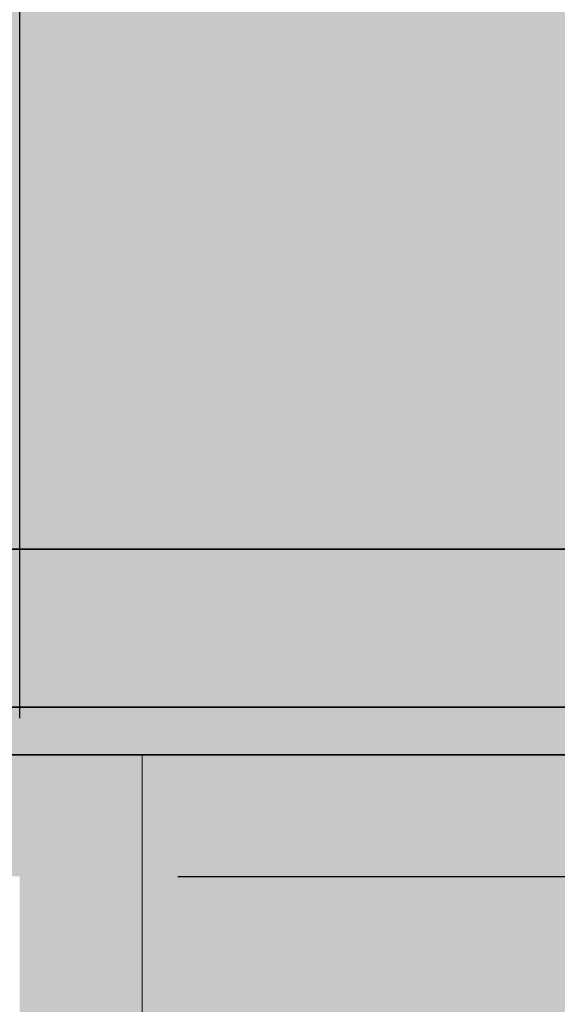
# Model space of a CAD drawing. Units: millimetres. Extents: x 130 to 1021, y 147 to 699.
# Tile 13 of 40: x 545 to 579, y 378 to 440. Entities that reach past the tile are written whole.
import ezdxf

# ---------------------------------------------------------------- set-up
doc = ezdxf.new("R2010")
doc.units = ezdxf.units.MM
doc.header["$MEASUREMENT"] = 0
for name, color, linetype, lineweight in [('A-ANNO-DIMS', 2, 'Continuous', 18), ('A-ELEV', 7, 'Continuous', 35), ('A-ELEV-PATT', 9, 'Continuous', 13), ('A-GLAZ', 4, 'Continuous', 18)]:
    doc.layers.add(name, color=color, linetype=linetype, lineweight=lineweight)
doc.styles.get("Standard").update_dxf_attribs({"font": 'arial.ttf'})
doc.dimstyles.get("Standard").update_dxf_attribs({"dimtxt": 20, "dimasz": 10, "dimexe": 10, "dimexo": 10, "dimgap": 5, "dimtad": 0, "dimtih": 1, "dimtoh": 1, "dimdec": 0, "dimzin": 0, "dimdsep": 46, "dimtxsty": 'Standard', "dimcen": 5, "dimadec": 0, "dimazin": 0, "dimtfac": 1, "dimtdec": 0, "dimtofl": 0, "dimtmove": 0, "dimatfit": 3, "dimfxl": 1, "dimtolj": 1, "dimtzin": 0, "dimarcsym": 0})

# ---------------------------------------------------------------- blocks, each defined once
blk = doc.blocks.new('*D7')
at = {"layer": 'A-ANNO-DIMS', "color": 0, "lineweight": -2, "transparency": 16777216}
for p, q in [((399.374, 349.447), (413.374, 349.447)), ((423.374, 349.447), (433.374, 349.447)), ((389.374, 344.547), (389.374, 339.447)), ((423.374, 344.547), (423.374, 339.447))]:
    blk.add_line(p, q, dxfattribs=at)
at = {"layer": 'A-ANNO-DIMS', "color": 0, "transparency": 16777216}
for points in [[(399.374, 351.114), (399.374, 347.781), (389.374, 349.447)], [(413.374, 351.114), (413.374, 347.781), (423.374, 349.447)]]:
    blk.add_solid(points, dxfattribs=at)
at = {"layer": 'Defpoints', "color": 0, "transparency": 16777216}
for p in [(389.374, 354.547), (423.374, 354.547), (423.374, 349.447)]:
    blk.add_point(p, dxfattribs=at)
at = {"layer": 'A-ANNO-DIMS', "color": 0, "transparency": 16777216, "insert": (582.037, 349.447), "char_height": 20, "attachment_point": 5}
blk.add_mtext('\\A1;DOOR PANEL 34 TYP.', dxfattribs=at)
blk = doc.blocks.new('*D11')
at = {"layer": 'A-ANNO-DIMS', "color": 0, "lineweight": -2, "transparency": 16777216}
for p, q in [((737.374, 648.699), (737.374, 149.739)), ((299.374, 566.947), (299.374, 149.739)), ((309.374, 159.739), (490.857, 159.739)), ((727.374, 159.739), (545.891, 159.739))]:
    blk.add_line(p, q, dxfattribs=at)
at = {"layer": 'A-ANNO-DIMS', "color": 0, "transparency": 16777216}
for points in [[(309.374, 161.406), (309.374, 158.073), (299.374, 159.739)], [(727.374, 161.406), (727.374, 158.073), (737.374, 159.739)]]:
    blk.add_solid(points, dxfattribs=at)
at = {"layer": 'Defpoints', "color": 0, "transparency": 16777216}
for p in [(737.374, 658.699), (299.374, 576.947), (737.374, 159.739)]:
    blk.add_point(p, dxfattribs=at)
at = {"layer": 'A-ANNO-DIMS', "color": 0, "transparency": 16777216, "insert": (518.374, 159.739), "char_height": 20, "attachment_point": 5}
blk.add_mtext('\\A1;438', dxfattribs=at)
blk = doc.blocks.new('*D22')
at = {"layer": 'A-ANNO-DIMS', "color": 0, "lineweight": -2, "transparency": 16777216}
for p, q in [((447.374, 656.947), (447.374, 696.247)), ((466.767, 403.947), (466.767, 696.247)), ((437.374, 686.247), (427.374, 686.247)), ((476.767, 686.247), (486.767, 686.247))]:
    blk.add_line(p, q, dxfattribs=at)
at = {"layer": 'A-ANNO-DIMS', "color": 0, "transparency": 16777216}
for points in [[(437.374, 687.914), (437.374, 684.581), (447.374, 686.247)], [(476.767, 687.914), (476.767, 684.581), (466.767, 686.247)]]:
    blk.add_solid(points, dxfattribs=at)
at = {"layer": 'Defpoints', "color": 0, "transparency": 16777216}
for p in [(466.767, 686.247), (447.374, 646.947), (466.767, 393.947)]:
    blk.add_point(p, dxfattribs=at)
at = {"layer": 'A-ANNO-DIMS', "color": 0, "transparency": 16777216, "insert": (532.34, 686.247), "char_height": 20, "attachment_point": 5}
blk.add_mtext('\\A1;19.393', dxfattribs=at)
blk = doc.blocks.new('*D23')
at = {"layer": 'A-ANNO-DIMS', "color": 0, "lineweight": -2, "transparency": 16777216}
for p, q in [((466.767, 403.947), (466.767, 696.247)), ((475.988, 209.039), (475.988, 696.247)), ((456.767, 686.247), (446.767, 686.247)), ((485.988, 686.247), (495.988, 686.247))]:
    blk.add_line(p, q, dxfattribs=at)
at = {"layer": 'A-ANNO-DIMS', "color": 0, "transparency": 16777216}
for points in [[(456.767, 687.914), (456.767, 684.581), (466.767, 686.247)], [(485.988, 687.914), (485.988, 684.581), (475.988, 686.247)]]:
    blk.add_solid(points, dxfattribs=at)
at = {"layer": 'Defpoints', "color": 0, "transparency": 16777216}
for p in [(475.988, 686.247), (466.767, 393.947), (475.988, 199.039)]:
    blk.add_point(p, dxfattribs=at)
at = {"layer": 'A-ANNO-DIMS', "color": 0, "transparency": 16777216, "insert": (534.631, 686.247), "char_height": 20, "attachment_point": 5}
blk.add_mtext('\\A1;9.222', dxfattribs=at)
blk = doc.blocks.new('*D24')
at = {"layer": 'A-ANNO-DIMS', "color": 0, "lineweight": -2, "transparency": 16777216}
for p, q in [((475.988, 209.039), (475.988, 696.247)), ((487.374, 671.947), (487.374, 696.247)), ((465.988, 686.247), (455.988, 686.247)), ((497.374, 686.247), (507.374, 686.247))]:
    blk.add_line(p, q, dxfattribs=at)
at = {"layer": 'A-ANNO-DIMS', "color": 0, "transparency": 16777216}
for points in [[(465.988, 687.914), (465.988, 684.581), (475.988, 686.247)], [(497.374, 687.914), (497.374, 684.581), (487.374, 686.247)]]:
    blk.add_solid(points, dxfattribs=at)
at = {"layer": 'Defpoints', "color": 0, "transparency": 16777216}
for p in [(487.374, 686.247), (487.374, 661.947), (475.988, 199.039)]:
    blk.add_point(p, dxfattribs=at)
at = {"layer": 'A-ANNO-DIMS', "color": 0, "transparency": 16777216, "insert": (553.022, 686.247), "char_height": 20, "attachment_point": 5}
blk.add_mtext('\\A1;11.385', dxfattribs=at)
blk = doc.blocks.new('*D27')
at = {"layer": 'A-ANNO-DIMS', "color": 0, "lineweight": -2, "transparency": 16777216}
for p, q in [((502.374, 593.947), (502.374, 696.247)), ((544.635, 396.264), (544.635, 696.247)), ((512.374, 686.247), (534.635, 686.247)), ((544.635, 686.247), (554.635, 686.247))]:
    blk.add_line(p, q, dxfattribs=at)
at = {"layer": 'A-ANNO-DIMS', "color": 0, "transparency": 16777216}
for points in [[(512.374, 687.914), (512.374, 684.581), (502.374, 686.247)], [(534.635, 687.914), (534.635, 684.581), (544.635, 686.247)]]:
    blk.add_solid(points, dxfattribs=at)
at = {"layer": 'Defpoints', "color": 0, "transparency": 16777216}
for p in [(544.635, 686.247), (502.374, 583.947), (544.635, 386.264)]:
    blk.add_point(p, dxfattribs=at)
at = {"layer": 'A-ANNO-DIMS', "color": 0, "transparency": 16777216, "insert": (593.776, 686.247), "char_height": 20, "attachment_point": 5}
blk.add_mtext('\\A1;42.26', dxfattribs=at)
blk = doc.blocks.new('*D28')
at = {"layer": 'A-ANNO-DIMS', "color": 0, "lineweight": -2, "transparency": 16777216}
for p, q in [((544.635, 396.264), (544.635, 696.247)), ((552.374, 593.947), (552.374, 696.247)), ((534.635, 686.247), (524.635, 686.247)), ((562.374, 686.247), (572.374, 686.247))]:
    blk.add_line(p, q, dxfattribs=at)
at = {"layer": 'A-ANNO-DIMS', "color": 0, "transparency": 16777216}
for points in [[(534.635, 687.914), (534.635, 684.581), (544.635, 686.247)], [(562.374, 687.914), (562.374, 684.581), (552.374, 686.247)]]:
    blk.add_solid(points, dxfattribs=at)
at = {"layer": 'Defpoints', "color": 0, "transparency": 16777216}
for p in [(552.374, 686.247), (552.374, 583.947), (544.635, 386.264)]:
    blk.add_point(p, dxfattribs=at)
at = {"layer": 'A-ANNO-DIMS', "color": 0, "transparency": 16777216, "insert": (611.057, 686.247), "char_height": 20, "attachment_point": 5}
blk.add_mtext('\\A1;7.738', dxfattribs=at)
blk = doc.blocks.new('*D51')
at = {"layer": 'A-ANNO-DIMS', "color": 0, "lineweight": -2, "transparency": 16777216}
for p, q in [((554.635, 386.264), (771.674, 386.264)), ((761.674, 376.264), (761.674, 348.674)), ((761.674, 290.662), (761.674, 318.251)), ((554.635, 280.662), (771.674, 280.662))]:
    blk.add_line(p, q, dxfattribs=at)
at = {"layer": 'A-ANNO-DIMS', "color": 0, "transparency": 16777216}
for points in [[(760.007, 376.264), (763.34, 376.264), (761.674, 386.264)], [(760.007, 290.662), (763.34, 290.662), (761.674, 280.662)]]:
    blk.add_solid(points, dxfattribs=at)
at = {"layer": 'Defpoints', "color": 0, "transparency": 16777216}
for p in [(544.635, 386.264), (761.674, 386.264), (544.635, 280.662)]:
    blk.add_point(p, dxfattribs=at)
at = {"layer": 'A-ANNO-DIMS', "color": 0, "transparency": 16777216, "insert": (761.674, 333.463), "char_height": 20, "attachment_point": 5}
blk.add_mtext('\\A1;105.6', dxfattribs=at)
blk = doc.blocks.new('*D52')
at = {"layer": 'A-ANNO-DIMS', "color": 0, "lineweight": -2, "transparency": 16777216}
for p, q in [((761.674, 403.947), (761.674, 413.947)), ((761.674, 413.947), (771.674, 413.947)), ((642.818, 393.947), (771.674, 393.947)), ((554.635, 386.264), (771.674, 386.264)), ((761.674, 376.264), (761.674, 366.264))]:
    blk.add_line(p, q, dxfattribs=at)
at = {"layer": 'A-ANNO-DIMS', "color": 0, "transparency": 16777216}
for points in [[(760.007, 403.947), (763.34, 403.947), (761.674, 393.947)], [(760.007, 376.264), (763.34, 376.264), (761.674, 386.264)]]:
    blk.add_solid(points, dxfattribs=at)
at = {"layer": 'Defpoints', "color": 0, "transparency": 16777216}
for p in [(632.818, 393.947), (761.674, 393.947), (544.635, 386.264)]:
    blk.add_point(p, dxfattribs=at)
at = {"layer": 'A-ANNO-DIMS', "color": 0, "transparency": 16777216, "insert": (810.337, 413.947), "char_height": 20, "attachment_point": 5}
blk.add_mtext('\\A1;7.683', dxfattribs=at)
blk = doc.blocks.new('*D54')
at = {"layer": 'A-ANNO-DIMS', "color": 0, "lineweight": -2, "transparency": 16777216}
for p, q in [((761.674, 473.947), (761.674, 483.947)), ((497.374, 463.947), (771.674, 463.947)), ((747.374, 403.69), (771.674, 403.69)), ((761.674, 393.69), (761.674, 383.69))]:
    blk.add_line(p, q, dxfattribs=at)
at = {"layer": 'A-ANNO-DIMS', "color": 0, "transparency": 16777216}
for points in [[(760.007, 473.947), (763.34, 473.947), (761.674, 463.947)], [(760.007, 393.69), (763.34, 393.69), (761.674, 403.69)]]:
    blk.add_solid(points, dxfattribs=at)
at = {"layer": 'Defpoints', "color": 0, "transparency": 16777216}
for p in [(487.374, 463.947), (761.674, 463.947), (737.374, 403.69)]:
    blk.add_point(p, dxfattribs=at)
at = {"layer": 'A-ANNO-DIMS', "color": 0, "transparency": 16777216, "insert": (761.674, 433.819), "char_height": 20, "attachment_point": 5}
blk.add_mtext('\\A1;60.26', dxfattribs=at)
blk = doc.blocks.new('*D65')
at = {"layer": 'A-ANNO-DIMS', "color": 0, "lineweight": -2, "transparency": 16777216}
for p, q in [((495.463, 509.127), (472.508, 423.108)), ((505.463, 509.127), (495.463, 509.127)), ((427.374, 248.979), (427.374, 258.979)), ((422.374, 253.979), (432.374, 253.979))]:
    blk.add_line(p, q, dxfattribs=at)
at = {"layer": 'A-ANNO-DIMS', "color": 0, "transparency": 16777216}
blk.add_solid([(470.898, 423.538), (474.118, 422.679), (469.93, 413.447)], dxfattribs=at)
at = {"layer": 'Defpoints', "color": 0, "transparency": 16777216}
for p in [(469.93, 413.447), (427.374, 253.979)]:
    blk.add_point(p, dxfattribs=at)
at = {"layer": 'A-ANNO-DIMS', "color": 0, "transparency": 16777216, "insert": (561.623, 509.127), "char_height": 20, "attachment_point": 5}
blk.add_mtext('\\A1;R165.05', dxfattribs=at)
blk = doc.blocks.new('*D67')
at = {"layer": 'A-ANNO-DIMS', "color": 0, "lineweight": -2, "transparency": 16777216}
for p, q in [((479.756, 492.431), (462.144, 412.223)), ((489.756, 492.431), (479.756, 492.431)), ((427.07, 247.496), (427.07, 257.496)), ((422.07, 252.496), (432.07, 252.496))]:
    blk.add_line(p, q, dxfattribs=at)
at = {"layer": 'A-ANNO-DIMS', "color": 0, "transparency": 16777216}
blk.add_solid([(460.516, 412.58), (463.772, 411.865), (459.999, 402.455)], dxfattribs=at)
at = {"layer": 'Defpoints', "color": 0, "transparency": 16777216}
for p in [(459.999, 402.455), (427.07, 252.496)]:
    blk.add_point(p, dxfattribs=at)
at = {"layer": 'A-ANNO-DIMS', "color": 0, "transparency": 16777216, "insert": (545.841, 492.431), "char_height": 20, "attachment_point": 5}
blk.add_mtext('\\A1;R153.53', dxfattribs=at)
blk = doc.blocks.new('*D69')
at = {"layer": 'A-ANNO-DIMS', "color": 0, "lineweight": -2, "transparency": 16777216}
for p, q in [((507.746, 572.261), (483.091, 501.813)), ((517.746, 572.261), (507.746, 572.261)), ((433.191, 354.23), (433.191, 364.23)), ((428.191, 359.23), (438.191, 359.23))]:
    blk.add_line(p, q, dxfattribs=at)
at = {"layer": 'A-ANNO-DIMS', "color": 0, "transparency": 16777216}
blk.add_solid([(481.518, 502.363), (484.664, 501.262), (479.788, 492.374)], dxfattribs=at)
at = {"layer": 'Defpoints', "color": 0, "transparency": 16777216}
for p in [(479.788, 492.374), (433.191, 359.23)]:
    blk.add_point(p, dxfattribs=at)
at = {"layer": 'A-ANNO-DIMS', "color": 0, "transparency": 16777216, "insert": (573.824, 572.261), "char_height": 20, "attachment_point": 5}
blk.add_mtext('\\A1;R141.06', dxfattribs=at)
blk = doc.blocks.new('*D71')
at = {"layer": 'A-ANNO-DIMS', "color": 0, "lineweight": -2, "transparency": 16777216}
for p, q in [((492.108, 581.609), (472.542, 512.666)), ((502.108, 581.609), (492.108, 581.609)), ((432.65, 367.109), (432.65, 377.109)), ((427.65, 372.109), (437.65, 372.109))]:
    blk.add_line(p, q, dxfattribs=at)
at = {"layer": 'A-ANNO-DIMS', "color": 0, "transparency": 16777216}
blk.add_solid([(470.938, 513.121), (474.145, 512.211), (469.812, 503.046)], dxfattribs=at)
at = {"layer": 'Defpoints', "color": 0, "transparency": 16777216}
for p in [(469.812, 503.046), (432.65, 372.109)]:
    blk.add_point(p, dxfattribs=at)
at = {"layer": 'A-ANNO-DIMS', "color": 0, "transparency": 16777216, "insert": (548.493, 581.609), "char_height": 20, "attachment_point": 5}
blk.add_mtext('\\A1;R136.1', dxfattribs=at)
blk = doc.blocks.new('*D72')
at = {"layer": 'A-ANNO-DIMS', "color": 0, "lineweight": -2, "transparency": 16777216}
for p, q in [((460.658, 573.64), (451.279, 503.49)), ((470.658, 573.64), (460.658, 573.64)), ((432.115, 355.142), (432.115, 365.142)), ((427.115, 360.142), (437.115, 360.142))]:
    blk.add_line(p, q, dxfattribs=at)
at = {"layer": 'A-ANNO-DIMS', "color": 0, "transparency": 16777216}
blk.add_solid([(449.628, 503.711), (452.931, 503.27), (449.954, 493.579)], dxfattribs=at)
at = {"layer": 'Defpoints', "color": 0, "transparency": 16777216}
for p in [(449.954, 493.579), (432.115, 360.142)]:
    blk.add_point(p, dxfattribs=at)
at = {"layer": 'A-ANNO-DIMS', "color": 0, "transparency": 16777216, "insert": (526.64, 573.64), "char_height": 20, "attachment_point": 5}
blk.add_mtext('\\A1;R134.62', dxfattribs=at)

msp = doc.modelspace()

# ---------------------------------------------------------------- hatches: boundary and pattern name
at = {"layer": 'A-ELEV-PATT'}
h = msp.add_hatch(color=256, dxfattribs=at)
h.dxf.hatch_style = 1
h.paths.add_polyline_path([(737.3738, 658.6988, 0.0135961), (632.4019, 661.9473), (607.3738, 661.9473), (487.3738, 661.9473), (487.3738, 649.9473), (607.3738, 649.9473), (632.3794, 649.9473, -0.0136841), (737.3738, 646.6784)])
h.paths.add_polyline_path([(732.3738, 643.9599, 0.0130529), (632.3738, 646.9473), (607.3738, 646.9473), (487.3738, 646.9473), (487.3738, 596.9473), (632.3738, 596.9473, -0.0130529), (732.3738, 593.9599)])
h.paths.add_polyline_path([(737.3738, 593.6732, 0.0137063), (632.3738, 596.9473), (487.3738, 596.9473), (487.3738, 586.9473), (632.355, 586.9473, -0.0137808), (737.3738, 583.6559)])
h.paths.add_polyline_path([(447.3738, 646.9473), (307.3738, 646.9473), (302.3738, 646.9473), (302.3738, 634.9473), (447.3738, 634.9473)])
h.paths.add_polyline_path([(447.3738, 631.9473), (307.3738, 631.9473), (307.3738, 586.9473), (447.3738, 586.9473)])
h.paths.add_polyline_path([(447.3738, 586.9473), (307.3738, 586.9473), (302.3738, 586.9473), (302.3738, 576.9473), (447.3738, 576.9473)])
h.paths.add_polyline_path([(447.3738, 573.9473), (367.3738, 573.9473), (367.3738, 539.9473), (447.3738, 539.9473)])
h.paths.add_polyline_path([(447.3738, 537.9473), (367.3738, 537.9473), (367.3738, 507.9473), (400.392, 507.4253, -0.001728), (401.3281, 507.6451, -0.5220025), (425.6117, 511.0391, -0.0391849), (447.3738, 510.4359), (447.3738, 510.7883)])
h.paths.add_polyline_path([(394.7238, 505.9473), (367.3738, 505.9473), (367.3738, 476.9473, -0.0146512), (375.8501, 480.2159), (376.1506, 499.2266, -0.0355419)])
h.paths.add_polyline_path([(632.3738, 583.9473), (552.3738, 583.9473), (552.3738, 550.9473), (632.3738, 550.9473)])
h.paths.add_polyline_path([(632.3738, 548.9473), (552.3738, 548.9473), (552.3738, 515.9473), (632.3738, 515.9473)])
h.paths.add_polyline_path([(632.3738, 513.9473), (552.3738, 513.9473), (552.3738, 476.9473), (632.3738, 476.9473)])
h.paths.add_polyline_path([(737.3738, 473.6903, 0.0136326), (632.3926, 476.9473), (552.3738, 476.9473), (487.3738, 476.9473), (487.3738, 466.9473), (632.3738, 466.9473, -0.0137063), (737.3738, 463.6732)])
h.paths.add_polyline_path([(732.3738, 460.9552, 0.0130741), (632.3681, 463.9473), (487.3738, 463.9473), (487.3738, 407.735, -0.0032286), (489.3544, 406.9473), (632.3926, 406.9473, -0.0129826), (732.3738, 403.9755)])
h.paths.add_polyline_path([(487.3738, 463.9473, 0.20133), (367.3738, 463.9473), (367.3738, 407.735, -0.1882031), (487.3738, 407.735)])
h.paths.add_polyline_path([(367.3738, 476.9473), (367.3738, 466.9473, -0.2013309), (487.3738, 466.9473), (487.3738, 476.9473, 0.20133)])
h.paths.add_polyline_path([(367.3738, 463.9473), (307.3738, 463.9473), (307.3738, 401.9473), (357.9413, 401.9473), (367.3738, 407.735)])
h.paths.add_polyline_path([(367.3738, 476.9473), (302.3738, 476.9473), (302.3738, 466.9473), (367.3738, 466.9473)])
h.paths.add_polyline_path([(632.8184, 366.9453), (552.3738, 366.9453), (552.3738, 393.9473), (632.8184, 393.9473)])
h.paths.add_polyline_path([(632.8184, 357.2114), (632.8184, 363.9453), (552.3738, 363.9453), (552.3738, 357.2114), (552.3738, 336.9453), (632.8184, 336.9453)])
h.paths.add_polyline_path([(632.8184, 333.9453), (552.3738, 333.9453), (552.3738, 306.9453), (632.8184, 306.9453)])
h.paths.add_polyline_path([(632.8184, 303.9453), (552.3738, 303.9453), (552.3738, 273.9473), (632.355, 273.9473, 0.0000608), (632.8184, 273.9491)])
h.paths.add_polyline_path([(737.3738, 403.6903, 0.0136326), (632.3926, 406.9473), (489.3544, 406.9473, 0.1915481), (367.3738, 407.735), (367.3738, 396.9473, -0.2013309), (487.3738, 396.9473), (632.3738, 396.9473, -0.0137063), (737.3738, 393.6732)])
h.paths.add_polyline_path([(357.9413, 401.9473), (307.3738, 401.9473), (307.3738, 391.9473), (357.9413, 391.9473)])
h.paths.add_polyline_path([(357.9413, 357.2114), (357.9413, 388.9473), (307.3738, 388.9473), (307.3738, 357.2114), (307.3738, 273.9473), (357.9413, 273.9473)])
h.paths.add_polyline_path([(732.3738, 263.93, -0.0130317), (632.3794, 260.9473), (466.7667, 260.9473), (466.7667, 240.9473), (469.8406, 236.978), (469.8406, 221.978), (472.9145, 218.0087), (472.9145, 213.9473), (607.3738, 213.9473), (732.3738, 213.9473)])
h.paths.add_polyline_path([(732.3738, 290.889), (722.479, 290.889), (722.479, 301.889), (732.3738, 301.889), (732.3738, 305.889), (722.479, 305.889), (722.479, 316.889), (732.3738, 316.889), (732.3738, 320.889), (722.479, 320.889), (722.479, 331.889), (732.3738, 331.889), (732.3738, 335.889), (722.479, 335.889), (722.479, 346.889), (732.3738, 346.889), (732.3738, 350.889), (722.479, 350.889), (722.479, 361.889), (732.3738, 361.889), (732.3738, 365.889), (722.479, 365.889), (722.479, 376.889), (732.3738, 376.889), (732.3738, 380.889), (722.479, 380.889), (722.479, 391.4848, 0.0005233), (718.479, 391.6843), (718.479, 380.889), (707.479, 380.889), (707.479, 392.1896, 0.0005231), (703.479, 392.3576), (703.479, 380.889), (692.479, 380.889), (692.479, 392.7765, 0.0005229), (688.479, 392.9131), (688.479, 380.889), (677.479, 380.889), (677.479, 393.2456, 0.0005228), (673.479, 393.3508), (673.479, 380.889), (662.479, 380.889), (662.479, 393.597, 0.0005227), (658.479, 393.6709), (658.479, 380.889), (647.479, 380.889), (647.479, 393.8308, 0.0005226), (643.479, 393.8732), (643.479, 380.889), (632.8184, 380.889), (632.8184, 376.889), (643.479, 376.889), (643.479, 365.889), (632.8184, 365.889), (632.8184, 361.889), (643.479, 361.889), (643.479, 350.889), (632.8184, 350.889), (632.8184, 346.889), (643.479, 346.889), (643.479, 335.889), (632.8184, 335.889), (632.8184, 331.889), (643.479, 331.889), (643.479, 320.889), (632.8184, 320.889), (632.8184, 316.889), (643.479, 316.889), (643.479, 305.889), (632.8184, 305.889), (632.8184, 301.889), (643.479, 301.889), (643.479, 290.889), (632.8184, 290.889), (632.8184, 286.889), (643.479, 286.889), (643.479, 274.0217, 0.0005246), (647.479, 274.0643), (647.479, 286.889), (658.479, 286.889), (658.479, 274.2248, 0.0005246), (662.479, 274.2989), (662.479, 286.889), (673.479, 286.889), (673.479, 274.546, 0.0005247), (677.479, 274.6516), (677.479, 286.889), (688.479, 286.889), (688.479, 274.9853, 0.0005248), (692.479, 275.1224), (692.479, 286.889), (703.479, 286.889), (703.479, 275.5429, 0.000525), (707.479, 275.7115), (707.479, 286.889), (718.479, 286.889), (718.479, 276.2187, 0.0005252), (722.479, 276.4189), (722.479, 286.889), (732.3738, 286.889)])
h.paths.add_polyline_path([(718.479, 290.889), (707.479, 290.889), (707.479, 301.889), (718.479, 301.889)], flags=16)
h.paths.add_polyline_path([(703.479, 290.889), (692.479, 290.889), (692.479, 301.889), (703.479, 301.889)], flags=16)
h.paths.add_polyline_path([(718.479, 305.889), (707.479, 305.889), (707.479, 316.889), (718.479, 316.889)], flags=16)
h.paths.add_polyline_path([(703.479, 305.889), (692.479, 305.889), (692.479, 316.889), (703.479, 316.889)], flags=16)
h.paths.add_polyline_path([(688.479, 290.889), (677.479, 290.889), (677.479, 301.889), (688.479, 301.889)], flags=16)
h.paths.add_polyline_path([(718.479, 320.889), (707.479, 320.889), (707.479, 331.889), (718.479, 331.889)], flags=16)
h.paths.add_polyline_path([(688.479, 305.889), (677.479, 305.889), (677.479, 316.889), (688.479, 316.889)], flags=16)
h.paths.add_polyline_path([(703.479, 320.889), (692.479, 320.889), (692.479, 331.889), (703.479, 331.889)], flags=16)
h.paths.add_polyline_path([(688.479, 320.889), (677.479, 320.889), (677.479, 331.889), (688.479, 331.889)], flags=16)
h.paths.add_polyline_path([(673.479, 290.889), (662.479, 290.889), (662.479, 301.889), (673.479, 301.889)], flags=16)
h.paths.add_polyline_path([(718.479, 335.889), (707.479, 335.889), (707.479, 346.889), (718.479, 346.889)], flags=16)
h.paths.add_polyline_path([(673.479, 305.889), (662.479, 305.889), (662.479, 316.889), (673.479, 316.889)], flags=16)
h.paths.add_polyline_path([(703.479, 335.889), (692.479, 335.889), (692.479, 346.889), (703.479, 346.889)], flags=16)
h.paths.add_polyline_path([(673.479, 320.889), (662.479, 320.889), (662.479, 331.889), (673.479, 331.889)], flags=16)
h.paths.add_polyline_path([(688.479, 335.889), (677.479, 335.889), (677.479, 346.889), (688.479, 346.889)], flags=16)
h.paths.add_polyline_path([(658.479, 290.889), (647.479, 290.889), (647.479, 301.889), (658.479, 301.889)], flags=16)
h.paths.add_polyline_path([(718.479, 350.889), (707.479, 350.889), (707.479, 361.889), (718.479, 361.889)], flags=16)
h.paths.add_polyline_path([(658.479, 305.889), (647.479, 305.889), (647.479, 316.889), (658.479, 316.889)], flags=16)
h.paths.add_polyline_path([(703.479, 350.889), (692.479, 350.889), (692.479, 361.889), (703.479, 361.889)], flags=16)
h.paths.add_polyline_path([(673.479, 335.889), (662.479, 335.889), (662.479, 346.889), (673.479, 346.889)], flags=16)
h.paths.add_polyline_path([(658.479, 320.889), (647.479, 320.889), (647.479, 331.889), (658.479, 331.889)], flags=16)
h.paths.add_polyline_path([(688.479, 350.889), (677.479, 350.889), (677.479, 361.889), (688.479, 361.889)], flags=16)
h.paths.add_polyline_path([(718.479, 365.889), (707.479, 365.889), (707.479, 376.889), (718.479, 376.889)], flags=16)
h.paths.add_polyline_path([(658.479, 335.889), (647.479, 335.889), (647.479, 346.889), (658.479, 346.889)], flags=16)
h.paths.add_polyline_path([(673.479, 350.889), (662.479, 350.889), (662.479, 361.889), (673.479, 361.889)], flags=16)
h.paths.add_polyline_path([(703.479, 365.889), (692.479, 365.889), (692.479, 376.889), (703.479, 376.889)], flags=16)
h.paths.add_polyline_path([(688.479, 365.889), (677.479, 365.889), (677.479, 376.889), (688.479, 376.889)], flags=16)
h.paths.add_polyline_path([(658.479, 350.889), (647.479, 350.889), (647.479, 361.889), (658.479, 361.889)], flags=16)
h.paths.add_polyline_path([(673.479, 365.889), (662.479, 365.889), (662.479, 376.889), (673.479, 376.889)], flags=16)
h.paths.add_polyline_path([(658.479, 365.889), (647.479, 365.889), (647.479, 376.889), (658.479, 376.889)], flags=16)
h.paths.add_polyline_path([(732.3738, 503.9786), (722.3392, 503.9786), (722.3392, 514.9786), (732.3738, 514.9786), (732.3738, 518.9786), (722.3392, 518.9786), (722.3392, 529.9786), (732.3738, 529.9786), (732.3738, 533.9786), (722.3392, 533.9786), (722.3392, 544.9786), (732.3738, 544.9786), (732.3738, 546.9473), (732.3738, 548.9786), (722.3392, 548.9786), (722.3392, 559.9786), (732.3738, 559.9786), (732.3738, 563.9786), (722.3392, 563.9786), (722.3392, 574.9786), (732.3738, 574.9786), (732.3738, 578.9786), (722.3392, 578.9786), (722.3392, 581.4789, 0.000526), (718.3392, 581.6791), (718.3392, 578.9786), (707.3392, 578.9786), (707.3392, 582.1863, 0.0005258), (703.3392, 582.355), (703.3392, 578.9786), (692.3392, 578.9786), (692.3392, 582.7752, 0.0005257), (688.3392, 582.9123), (688.3392, 578.9786), (677.3392, 578.9786), (677.3392, 583.2457, 0.0005255), (673.3392, 583.3512), (673.3392, 578.9786), (662.3392, 578.9786), (662.3392, 583.5978, 0.0005254), (658.3392, 583.6718), (658.3392, 578.9786), (647.3392, 578.9786), (647.3392, 583.8317, 0.0005254), (643.3392, 583.8741), (643.3392, 578.9786), (632.3738, 578.9786), (632.3738, 574.9786), (643.3392, 574.9786), (643.3392, 563.9786), (632.3738, 563.9786), (632.3738, 559.9786), (643.3392, 559.9786), (643.3392, 548.9786), (632.3738, 548.9786), (632.3738, 544.9786), (643.3392, 544.9786), (643.3392, 533.9786), (632.3738, 533.9786), (632.3738, 529.9786), (643.3392, 529.9786), (643.3392, 518.9786), (632.3738, 518.9786), (632.3738, 515.9473), (632.3738, 514.9786), (643.3392, 514.9786), (643.3392, 503.9786), (632.3738, 503.9786), (632.3738, 499.9786), (643.3392, 499.9786), (643.3392, 488.9786), (632.3738, 488.9786), (632.3738, 484.9786), (643.3392, 484.9786), (643.3392, 476.8751, -0.0005191), (647.3392, 476.8332), (647.3392, 484.9786), (658.3392, 484.9786), (658.3392, 476.6752, -0.0005192), (662.3392, 476.6022), (662.3392, 484.9786), (673.3392, 484.9786), (673.3392, 476.3585, -0.0005193), (677.3392, 476.2543), (677.3392, 484.9786), (688.3392, 484.9786), (688.3392, 475.9248, -0.0005194), (692.3392, 475.7894), (692.3392, 484.9786), (703.3392, 484.9786), (703.3392, 475.3741, -0.0005195), (707.3392, 475.2075), (707.3392, 484.9786), (718.3392, 484.9786), (718.3392, 474.7064, -0.0005197), (722.3392, 474.5086), (722.3392, 484.9786), (732.3738, 484.9786), (732.3738, 488.9786), (722.3392, 488.9786), (722.3392, 499.9786), (732.3738, 499.9786)])
h.paths.add_polyline_path([(718.3392, 503.9786), (707.3392, 503.9786), (707.3392, 514.9786), (718.3392, 514.9786)], flags=16)
h.paths.add_polyline_path([(718.3392, 499.9786), (718.3392, 488.9786), (707.3392, 488.9786), (707.3392, 499.9786)], flags=16)
h.paths.add_polyline_path([(718.3392, 518.9786), (707.3392, 518.9786), (707.3392, 529.9786), (718.3392, 529.9786)], flags=16)
h.paths.add_polyline_path([(703.3392, 503.9786), (692.3392, 503.9786), (692.3392, 514.9786), (703.3392, 514.9786)], flags=16)
h.paths.add_polyline_path([(703.3392, 499.9786), (703.3392, 488.9786), (692.3392, 488.9786), (692.3392, 499.9786)], flags=16)
h.paths.add_polyline_path([(703.3392, 518.9786), (692.3392, 518.9786), (692.3392, 529.9786), (703.3392, 529.9786)], flags=16)
h.paths.add_polyline_path([(718.3392, 533.9786), (707.3392, 533.9786), (707.3392, 544.9786), (718.3392, 544.9786)], flags=16)
h.paths.add_polyline_path([(688.3392, 503.9786), (677.3392, 503.9786), (677.3392, 514.9786), (688.3392, 514.9786)], flags=16)
h.paths.add_polyline_path([(688.3392, 499.9786), (688.3392, 488.9786), (677.3392, 488.9786), (677.3392, 499.9786)], flags=16)
h.paths.add_polyline_path([(703.3392, 533.9786), (692.3392, 533.9786), (692.3392, 544.9786), (703.3392, 544.9786)], flags=16)
h.paths.add_polyline_path([(688.3392, 518.9786), (677.3392, 518.9786), (677.3392, 529.9786), (688.3392, 529.9786)], flags=16)
h.paths.add_polyline_path([(688.3392, 533.9786), (677.3392, 533.9786), (677.3392, 544.9786), (688.3392, 544.9786)], flags=16)
h.paths.add_polyline_path([(718.3392, 548.9786), (707.3392, 548.9786), (707.3392, 559.9786), (718.3392, 559.9786)], flags=16)
h.paths.add_polyline_path([(673.3392, 503.9786), (662.3392, 503.9786), (662.3392, 514.9786), (673.3392, 514.9786)], flags=16)
h.paths.add_polyline_path([(673.3392, 499.9786), (673.3392, 488.9786), (662.3392, 488.9786), (662.3392, 499.9786)], flags=16)
h.paths.add_polyline_path([(703.3392, 548.9786), (692.3392, 548.9786), (692.3392, 559.9786), (703.3392, 559.9786)], flags=16)
h.paths.add_polyline_path([(673.3392, 518.9786), (662.3392, 518.9786), (662.3392, 529.9786), (673.3392, 529.9786)], flags=16)
h.paths.add_polyline_path([(688.3392, 548.9786), (677.3392, 548.9786), (677.3392, 559.9786), (688.3392, 559.9786)], flags=16)
h.paths.add_polyline_path([(673.3392, 533.9786), (662.3392, 533.9786), (662.3392, 544.9786), (673.3392, 544.9786)], flags=16)
h.paths.add_polyline_path([(718.3392, 563.9786), (707.3392, 563.9786), (707.3392, 574.9786), (718.3392, 574.9786)], flags=16)
h.paths.add_polyline_path([(658.3392, 503.9786), (647.3392, 503.9786), (647.3392, 514.9786), (658.3392, 514.9786)], flags=16)
h.paths.add_polyline_path([(658.3392, 499.9786), (658.3392, 488.9786), (647.3392, 488.9786), (647.3392, 499.9786)], flags=16)
h.paths.add_polyline_path([(703.3392, 563.9786), (692.3392, 563.9786), (692.3392, 574.9786), (703.3392, 574.9786)], flags=16)
h.paths.add_polyline_path([(658.3392, 518.9786), (647.3392, 518.9786), (647.3392, 529.9786), (658.3392, 529.9786)], flags=16)
h.paths.add_polyline_path([(673.3392, 548.9786), (662.3392, 548.9786), (662.3392, 559.9786), (673.3392, 559.9786)], flags=16)
h.paths.add_polyline_path([(688.3392, 563.9786), (677.3392, 563.9786), (677.3392, 574.9786), (688.3392, 574.9786)], flags=16)
h.paths.add_polyline_path([(658.3392, 533.9786), (647.3392, 533.9786), (647.3392, 544.9786), (658.3392, 544.9786)], flags=16)
h.paths.add_polyline_path([(673.3392, 563.9786), (662.3392, 563.9786), (662.3392, 574.9786), (673.3392, 574.9786)], flags=16)
h.paths.add_polyline_path([(658.3392, 548.9786), (647.3392, 548.9786), (647.3392, 559.9786), (658.3392, 559.9786)], flags=16)
h.paths.add_polyline_path([(658.3392, 563.9786), (647.3392, 563.9786), (647.3392, 574.9786), (658.3392, 574.9786)], flags=16)
h = msp.add_hatch(color=256, dxfattribs=at)
h.dxf.hatch_style = 1
h.paths.add_polyline_path([(447.3738, 576.9473), (302.3738, 576.9473), (302.3738, 573.9473), (447.3738, 573.9473)])
h.paths.add_polyline_path([(487.3738, 583.9473), (487.3738, 586.9473), (447.3738, 576.9473), (447.3738, 573.9473)])
h.paths.add_polyline_path([(632.355, 586.9473), (487.3738, 586.9473), (487.3738, 583.9473), (632.3738, 583.9473), (632.3738, 583.9472, -0.0138), (737.3738, 580.6507), (737.3738, 583.6559, 0.0137808)])
h.paths.add_polyline_path([(367.3738, 466.9473), (302.3738, 466.9473), (302.3738, 463.9473), (367.3738, 463.9473)])
h.paths.add_polyline_path([(487.3738, 463.9473), (487.3738, 466.9473, 0.2013309), (367.3738, 466.9473), (367.3738, 463.9473, -0.20133)])
h.paths.add_polyline_path([(632.3738, 466.9473), (487.3738, 466.9473), (487.3738, 463.9473), (632.3681, 463.9473, -0.0137285), (737.3738, 460.6681), (737.3738, 463.6732, 0.0137063)])
h.paths.add_polyline_path([(632.3738, 396.9473), (487.3738, 396.9473, 0.2013309), (367.3738, 396.9473), (367.3738, 393.9473, -0.2023717), (486.7667, 393.9473), (632.3681, 393.9473, -0.0137285), (737.3738, 390.6681), (737.3738, 393.6732, 0.0137063)])
h.paths.add_polyline_path([(357.9413, 391.9473), (307.3738, 391.9473), (307.3738, 388.9473), (357.9413, 388.9473)])
h.paths.add_polyline_path([(367.3738, 393.9473), (367.3738, 396.9473), (357.9413, 391.924), (357.9413, 388.9473), (358.058, 388.9473)])
h.paths.add_polyline_path([(737.3738, 264.2162), (737.3738, 267.2214, -0.0137063), (632.3738, 263.9473), (463.7667, 263.9473), (466.7667, 260.9473), (632.3794, 260.9473, 0.0136841)])
h.paths.add_polyline_path([(463.7667, 263.9473), (447.3738, 263.9473), (450.3738, 260.9473), (466.7667, 260.9473)])
h.paths.add_polyline_path([(447.3738, 263.9473), (432.3738, 263.9473), (432.3738, 260.9473), (450.3738, 260.9473)])
h.paths.add_polyline_path([(382.3738, 263.9473), (357.9413, 263.9473), (357.9413, 260.9473), (382.3738, 260.9473)])
h.paths.add_polyline_path([(357.9413, 263.9473), (307.3738, 263.9473), (307.3738, 260.9473), (357.9413, 260.9473)])
h = msp.add_hatch(color=256, dxfattribs=at)
h.paths.add_polyline_path([(327.3738, 569.884), (327.3738, 573.9473), (307.3738, 573.9473), (307.3738, 476.9473), (327.3738, 476.9473), (327.3738, 480.95)])
h.paths.add_polyline_path([(486.7667, 386.2639), (486.7667, 393.9473), (466.7667, 393.9473), (466.7667, 357.2114), (466.7667, 311.9335, 0.0342703), (486.7667, 308.4637)])
h.paths.add_polyline_path([(486.7667, 308.4637, -0.0342703), (466.7667, 311.9335), (466.7667, 273.9473), (486.7667, 273.9473)])
h.paths.add_polyline_path([(389.3738, 351.5473), (396.7693, 351.5473, -0.007027), (393.8774, 354.5473), (389.3738, 354.5473), (389.3738, 359.5775, -0.0190302), (382.3738, 368.424), (382.3738, 249.5473), (432.3738, 249.5473), (432.3738, 325.067, -0.0057673), (429.3738, 326.709), (429.3738, 257.5473), (426.3738, 257.5473), (426.3738, 328.4428, -0.0059254), (423.3738, 330.272), (423.3738, 315.7473), (389.3738, 315.7473), (389.3738, 332.1473), (420.4552, 332.1473, -0.008951), (416.0768, 335.1473), (389.3738, 335.1473)])
h.paths.add_polyline_path([(389.3738, 312.7473), (423.3738, 312.7473), (423.3738, 296.3473), (389.3738, 296.3473)], flags=16)
h.paths.add_polyline_path([(389.3738, 293.3473), (423.3738, 293.3473), (423.3738, 276.9473), (389.3738, 276.9473)], flags=16)
h.paths.add_polyline_path([(389.3738, 273.9473), (423.3738, 273.9473), (423.3738, 257.5473), (389.3738, 257.5473)], flags=16)
h.paths.add_polyline_path([(432.3738, 378.9473), (382.3738, 378.9473), (382.3738, 368.424, 0.0190302), (389.3738, 359.5775), (389.3738, 370.9473), (423.3738, 370.9473), (423.3738, 354.5473), (393.8774, 354.5473, 0.007027), (396.7693, 351.5473), (423.3738, 351.5473), (423.3738, 335.1473), (416.0768, 335.1473, 0.008951), (420.4552, 332.1473), (423.3738, 332.1473), (423.3738, 330.272, 0.0059254), (426.3738, 328.4428), (426.3738, 370.9473), (429.3738, 370.9473), (429.3738, 326.709, 0.0057673), (432.3738, 325.067)])
h.paths.add_polyline_path([(466.7667, 357.2114), (466.7667, 393.9473), (447.3738, 393.9473), (447.3738, 357.2114), (447.3738, 318.1243, 0.0063261), (450.8779, 316.785), (450.8779, 331.5915), (463.5608, 331.5915), (463.5608, 312.7571, 0.005582), (466.7667, 311.9335)])
h.paths.add_polyline_path([(450.8779, 334.5915), (450.8779, 360.0915), (463.5608, 360.0915), (463.5608, 334.5915)], flags=16)
h.paths.add_polyline_path([(450.8779, 363.0915), (450.8779, 388.6449), (463.5608, 388.6449), (463.5608, 363.0915)], flags=16)
h.paths.add_polyline_path([(466.7667, 311.9335, -0.005582), (463.5608, 312.7571), (463.5608, 306.0915), (450.8779, 306.0915), (450.8779, 316.785, -0.0063261), (447.3738, 318.1243), (447.3738, 273.9473), (466.7667, 273.9473)])
h.paths.add_polyline_path([(450.8779, 303.0915), (463.5608, 303.0915), (463.5608, 277.5915), (450.8779, 277.5915)], flags=16)
h.paths.add_polyline_path([(552.3738, 357.2114), (552.3738, 393.9473), (486.7667, 393.9473), (486.7667, 386.2639), (544.6354, 386.2639), (544.6354, 280.6619), (486.7667, 280.6619), (486.7667, 273.9473), (552.3738, 273.9473)])
h.paths.add_polyline_path([(487.3738, 583.9473), (472.3738, 580.1973), (472.3738, 507.0765), (472.3738, 505.4251, -0.0056452), (475.3738, 504.4942), (475.3738, 506.3543), (475.3738, 511.9473), (484.3738, 511.9473), (484.3738, 503.8134), (484.3738, 501.2439, -0.0058357), (487.3738, 500.0015)])
h.paths.add_polyline_path([(484.3738, 578.0434), (484.3738, 548.9473), (475.3738, 548.9473), (475.3738, 575.7934)], flags=16)
h.paths.add_polyline_path([(484.3738, 546.9473), (484.3738, 513.9473), (475.3738, 513.9473), (475.3738, 518.7148), (475.3738, 546.9473)], flags=16)

# ---------------------------------------------------------------- linework, layer by layer
at = {"layer": 'A-ELEV'}
for p, q in [((632.3738, 406.9473), (489.3544, 406.9473)), ((632.3738, 396.9473), (487.3738, 396.9473)), ((632.3738, 393.9473), (367.3738, 393.9473))]:
    msp.add_line(p, q, dxfattribs=at)
at = {"layer": 'A-GLAZ'}
msp.add_line((552.3738, 393.9473), (552.3738, 357.2114), dxfattribs=at)

# ---------------------------------------------------------------- dimensions: what is measured, and where the dimension line sits
at = {"layer": 'A-ANNO-DIMS'}
for base, p1, p2, override, picture, middle in [((466.7667, 686.2473), (447.3738, 646.9473), (466.7667, 393.9473), {"dimdec": 3, "dimlfac": 1, "dimrnd": 0, "dimzin": 0, "dimdsep": 46, "dimlunit": 2}, '*D22', (532.3397, 686.2473)), ((475.9885, 686.2473), (466.7667, 393.9473), (475.9885, 199.0395), {"dimdec": 3, "dimlfac": 1, "dimrnd": 0, "dimzin": 0, "dimdsep": 46, "dimlunit": 2}, '*D23', (534.631, 686.2473)), ((487.3738, 686.2473), (475.9885, 199.0395), (487.3738, 661.9473), {"dimdec": 3, "dimlfac": 1, "dimrnd": 0, "dimzin": 0, "dimdsep": 46, "dimlunit": 2}, '*D24', (553.0218, 686.2473)), ((544.6354, 686.2473), (502.3738, 583.9473), (544.6354, 386.2639), {"dimdec": 2, "dimlfac": 1, "dimrnd": 0, "dimzin": 0, "dimdsep": 46, "dimlunit": 2}, '*D27', (593.776, 686.2473)), ((552.3738, 686.2473), (544.6354, 386.2639), (552.3738, 583.9473), {"dimdec": 3, "dimlfac": 1, "dimrnd": 0, "dimzin": 0, "dimdsep": 46, "dimlunit": 2}, '*D28', (611.0573, 686.2473)), ((737.3738, 159.7395), (299.3738, 576.9473), (737.3738, 658.6988), {"dimdec": 0, "dimlfac": 1, "dimrnd": 0, "dimzin": 0, "dimdsep": 46, "dimlunit": 2}, '*D11', (518.3738, 159.7395))]:
    dim = msp.add_linear_dim(base=base, p1=p1, p2=p2, dimstyle='Standard', override=override, dxfattribs=at)
    dim.commit()
    dim.dimension.update_dxf_attribs({"geometry": picture, "text_midpoint": middle})
for center, mpoint, override, picture, middle in [((432.6505, 372.1087), (469.8116, 503.0461), {"dimdec": 1, "dimlfac": 1, "dimrnd": 0, "dimzin": 0, "dimdsep": 46, "dimlunit": 2}, '*D71', (548.493, 581.6085)), ((432.115, 360.1423), (449.9544, 493.5786), {"dimdec": 2, "dimlfac": 1, "dimrnd": 0, "dimzin": 0, "dimdsep": 46, "dimlunit": 2}, '*D72', (526.6403, 573.6404)), ((433.1906, 359.2304), (479.788, 492.3743), {"dimdec": 2, "dimlfac": 1, "dimrnd": 0, "dimzin": 0, "dimdsep": 46, "dimlunit": 2}, '*D69', (573.8242, 572.2606)), ((427.3738, 253.9788), (469.9297, 413.4465), {"dimdec": 2, "dimlfac": 1, "dimrnd": 0, "dimzin": 0, "dimdsep": 46, "dimlunit": 2}, '*D65', (561.6228, 509.1272)), ((427.0702, 252.4956), (459.999, 402.4554), {"dimdec": 2, "dimlfac": 1, "dimrnd": 0, "dimzin": 0, "dimdsep": 46, "dimlunit": 2}, '*D67', (545.8408, 492.4313))]:
    dim = msp.add_radius_dim(center=center, mpoint=mpoint, dimstyle='Standard', override=override, dxfattribs=at)
    dim.commit()
    dim.dimension.update_dxf_attribs({"geometry": picture, "text_midpoint": middle, "dimtype": 164})
for base, p1, p2, override, picture, middle in [((761.6738, 463.9473), (737.3738, 403.6903), (487.3738, 463.9473), {"dimdec": 2, "dimlfac": 1, "dimrnd": 0, "dimzin": 0, "dimdsep": 46, "dimlunit": 2}, '*D54', (761.6738, 433.8188)), ((761.6738, 393.9473), (544.6354, 386.2639), (632.8184, 393.9473), {"dimdec": 3, "dimlfac": 1, "dimrnd": 0, "dimzin": 0, "dimdsep": 46, "dimlunit": 2}, '*D52', (810.3368, 413.9473)), ((761.6738, 386.2639), (544.6354, 280.6619), (544.6354, 386.2639), {"dimdec": 1, "dimlfac": 1, "dimrnd": 0, "dimzin": 0, "dimdsep": 46, "dimlunit": 2}, '*D51', (761.6738, 333.4629))]:
    dim = msp.add_linear_dim(base=base, p1=p1, p2=p2, angle=90, dimstyle='Standard', override=override, dxfattribs=at)
    dim.commit()
    dim.dimension.update_dxf_attribs({"geometry": picture, "text_midpoint": middle})
dim = msp.add_linear_dim(base=(423.3738, 349.4473), p1=(389.3738, 354.5473), p2=(423.3738, 354.5473), text='DOOR PANEL <> TYP.', dimstyle='Standard', override={"dimdec": 0, "dimrnd": 0, "dimzin": 0, "dimlunit": 2}, dxfattribs=at)
dim.commit()
dim.dimension.update_dxf_attribs({"geometry": '*D7', "text_midpoint": (582.0368, 349.4473)})

doc.saveas('drawing.dxf')
